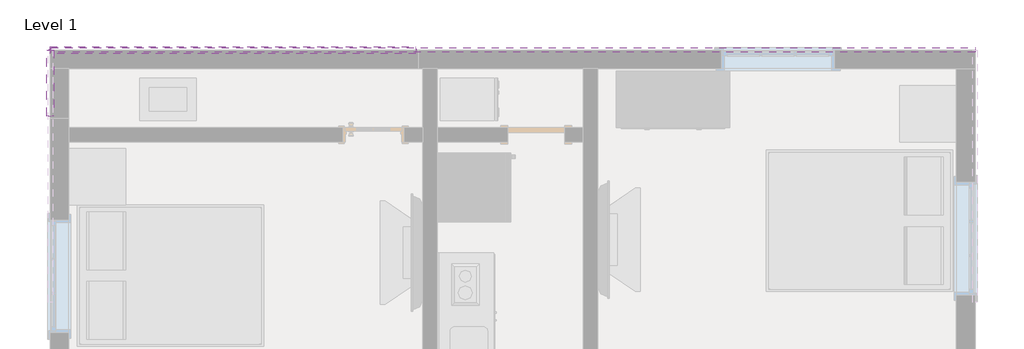
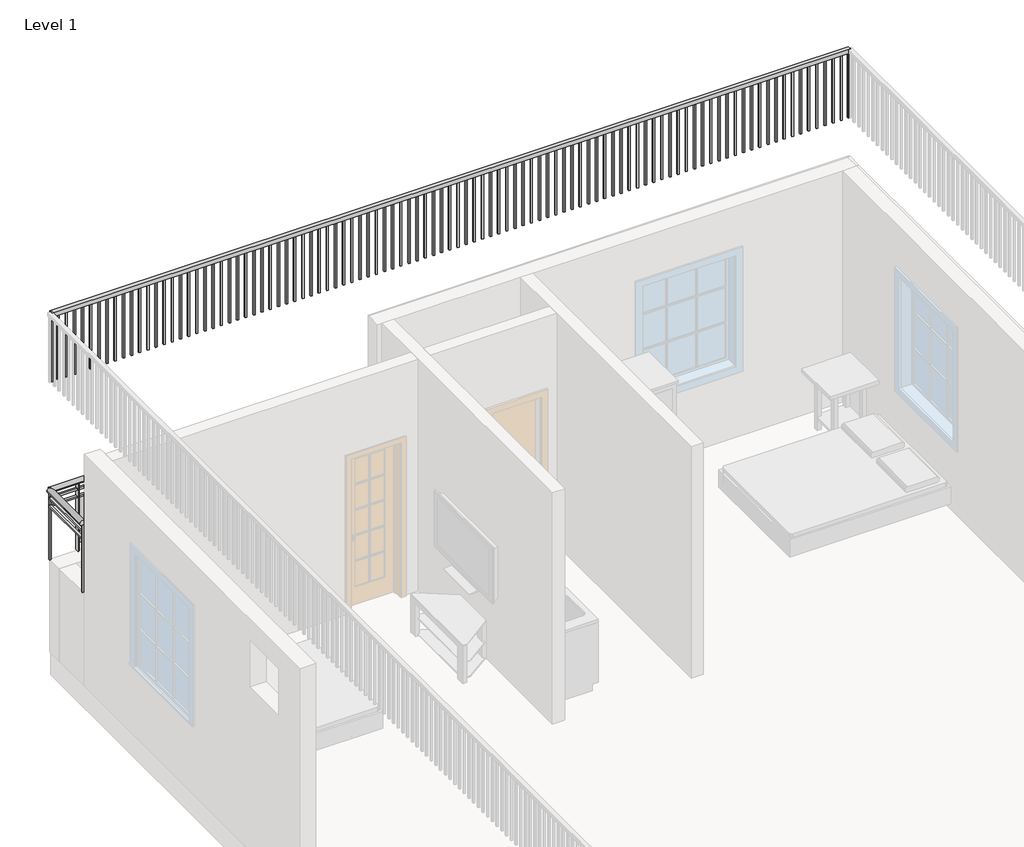
# One storey, part 5 of 7: 3 railings.
"""IFC4 building model written with IfcOpenShell, lengths in millimetres."""

from ifc_helpers import new_model, si_unit, point, frame, origin, place, context, project, spatial, polyline, ellipse_curve, trimmed, outline, extrude, element, save
from ifc_brep_helpers import plane_surface, extruded_surface, advanced_brep

model = new_model("IFC4")

# Units and contexts
model_context = context("Model", 3, world=origin())
ifc_project = project(units=[si_unit("LENGTHUNIT", "METRE", prefix="MILLI")], contexts=[model_context])

# Site, building, storey
site = spatial("IfcSite", under=ifc_project)
building = spatial("IfcBuilding", under=site)
storey = spatial("IfcBuildingStorey", under=building, Name="Level 1", Elevation=0.0)

# Railings
placement = place(None, origin())
element("IfcRailing", 1, ObjectType="Glass Panel - Bottom Fill", at=placement, inside=storey, context=model_context, shape_type="SolidModel", body=[
    advanced_brep(
    [(-4543.28475, 12412.5839473, 2133.6), (-4543.28475, 12488.7839473, 2133.6), (-8480.28475, 12412.5839473, 2133.6), (-8480.28475, 12488.7839473, 2133.6)],
    [
        (0, 1, ellipse_curve(frame((-4543.28475, 12450.6839473, 2133.6), z_axis=(1.0, 0.0, 0.0), x_axis=(0.0, 1.0, 0.0)), 38.1, 28.575)),
        (1, 0, ellipse_curve(frame((-4543.28475, 12450.6839473, 2133.6), z_axis=(1.0, 0.0, 0.0), x_axis=(0.0, 1.0, 0.0)), 38.1, 28.575)),
        (2, 3, ellipse_curve(frame((-8480.28475, 12450.6839473, 2133.6), z_axis=(-1.0, 0.0, 0.0), x_axis=(0.0, 1.0, 0.0)), 38.1, 28.575)),
        (3, 2, ellipse_curve(frame((-8480.28475, 12450.6839473, 2133.6), z_axis=(-1.0, 0.0, 0.0), x_axis=(0.0, 1.0, 0.0)), 38.1, 28.575)),
        (0, 2),
        (3, 1),
    ],
    [
        plane_surface(frame((-4543.28475, 12450.6839473, 2133.6), z_axis=(1.0, 0.0, 0.0), x_axis=(0.0, -1.0, 0.0))),
        plane_surface(frame((-8480.28475, 12450.6839473, 2133.6), z_axis=(-1.0, 0.0, 0.0), x_axis=(0.0, -1.0, 0.0))),
        extruded_surface(trimmed(ellipse_curve(frame((-8480.28475, 12450.6839473, 2133.6), z_axis=(1.0, 0.0, 0.0), x_axis=(0.0, 1.0, 0.0)), 38.1, 28.575), [point((-8480.28475, 12412.5839473, 2133.6))], [point((-8480.28475, 12488.7839473, 2133.6))], True, "CARTESIAN"), (3937.000000000001, 0.0, 0.0), 3937.000000000001),
        extruded_surface(trimmed(ellipse_curve(frame((-8480.28475, 12450.6839473, 2133.6), z_axis=(1.0, 0.0, 0.0), x_axis=(0.0, 1.0, 0.0)), 38.1, 28.575), [point((-8480.28475, 12488.7839473, 2133.6))], [point((-8480.28475, 12412.5839473, 2133.6))], True, "CARTESIAN"), (3937.000000000001, 0.0, 0.0), 3937.000000000001),
    ],
    [
        (0, [[1, 2]]),
        (1, [[3, 4]]),
        (2, [[-1, 5, -4, 6]]),
        (3, [[-2, -6, -3, -5]]),
    ],
),
    extrude(outline(polyline([(-4543.28475, 12463.3839473), (-4543.28475, 12437.9839473), (-8480.28475, 12437.9839473), (-8480.28475, 12463.3839473), (-4543.28475, 12463.3839473)])), frame((0.0, 0.0, 2019.3), z_axis=(0.0, 0.0, 1.0), x_axis=(1.0, 0.0, 0.0)), (0.0, 0.0, 1.0), 25.4),
    extrude(outline(polyline([(-4543.28475, 12463.3839473), (-4543.28475, 12437.9839473), (-8480.28475, 12437.9839473), (-8480.28475, 12463.3839473), (-4543.28475, 12463.3839473)])), frame((0.0, 0.0, 1917.7), z_axis=(0.0, 0.0, 1.0), x_axis=(1.0, 0.0, 0.0)), (0.0, 0.0, 1.0), 25.4),
    extrude(outline(polyline([(-8131.03475, 12476.0839473), (-8131.03475, 12425.2839473), (-8143.73475, 12425.2839473), (-8143.73475, 12476.0839473), (-8131.03475, 12476.0839473)])), frame((0.0, 0.0, 1219.2), z_axis=(0.0, 0.0, 1.0), x_axis=(1.0, 0.0, 0.0)), (0.0, 0.0, 1.0), 885.6788223),
    extrude(outline(polyline([(-7324.58475, 12444.1487903), (-8137.38475, 12444.1487903), (-8137.38475, 12450.4987903), (-7324.58475, 12450.4987903), (-7324.58475, 12444.1487903)])), frame((0.0, 0.0, 1320.8), z_axis=(0.0, 0.0, 1.0), x_axis=(1.0, 0.0, 0.0)), (0.0, 0.0, 1.0), 596.9),
    extrude(outline(polyline([(-7318.23475, 12476.0839473), (-7318.23475, 12425.2839473), (-7330.93475, 12425.2839473), (-7330.93475, 12476.0839473), (-7318.23475, 12476.0839473)])), frame((0.0, 0.0, 1219.2), z_axis=(0.0, 0.0, 1.0), x_axis=(1.0, 0.0, 0.0)), (0.0, 0.0, 1.0), 885.6788223),
    extrude(outline(polyline([(-6511.78475, 12444.1487903), (-7324.58475, 12444.1487903), (-7324.58475, 12450.4987903), (-6511.78475, 12450.4987903), (-6511.78475, 12444.1487903)])), frame((0.0, 0.0, 1320.8), z_axis=(0.0, 0.0, 1.0), x_axis=(1.0, 0.0, 0.0)), (0.0, 0.0, 1.0), 596.9),
    extrude(outline(polyline([(-6505.43475, 12476.0839473), (-6505.43475, 12425.2839473), (-6518.13475, 12425.2839473), (-6518.13475, 12476.0839473), (-6505.43475, 12476.0839473)])), frame((0.0, 0.0, 1219.2), z_axis=(0.0, 0.0, 1.0), x_axis=(1.0, 0.0, 0.0)), (0.0, 0.0, 1.0), 885.6788223),
    extrude(outline(polyline([(-5698.98475, 12444.1487903), (-6511.78475, 12444.1487903), (-6511.78475, 12450.4987903), (-5698.98475, 12450.4987903), (-5698.98475, 12444.1487903)])), frame((0.0, 0.0, 1320.8), z_axis=(0.0, 0.0, 1.0), x_axis=(1.0, 0.0, 0.0)), (0.0, 0.0, 1.0), 596.9),
    extrude(outline(polyline([(-5692.63475, 12476.0839473), (-5692.63475, 12425.2839473), (-5705.33475, 12425.2839473), (-5705.33475, 12476.0839473), (-5692.63475, 12476.0839473)])), frame((0.0, 0.0, 1219.2), z_axis=(0.0, 0.0, 1.0), x_axis=(1.0, 0.0, 0.0)), (0.0, 0.0, 1.0), 885.6788223),
    extrude(outline(polyline([(-4886.18475, 12444.1487903), (-5698.98475, 12444.1487903), (-5698.98475, 12450.4987903), (-4886.18475, 12450.4987903), (-4886.18475, 12444.1487903)])), frame((0.0, 0.0, 1320.8), z_axis=(0.0, 0.0, 1.0), x_axis=(1.0, 0.0, 0.0)), (0.0, 0.0, 1.0), 596.9),
    extrude(outline(polyline([(-4879.83475, 12476.0839473), (-4879.83475, 12425.2839473), (-4892.53475, 12425.2839473), (-4892.53475, 12476.0839473), (-4879.83475, 12476.0839473)])), frame((0.0, 0.0, 1219.2), z_axis=(0.0, 0.0, 1.0), x_axis=(1.0, 0.0, 0.0)), (0.0, 0.0, 1.0), 885.6788223),
    extrude(outline(polyline([(-8467.58475, 12460.2089473), (-8467.58475, 12441.1589473), (-8486.63475, 12441.1589473), (-8486.63475, 12460.2089473), (-8467.58475, 12460.2089473)])), frame((0.0, 0.0, 1219.2), z_axis=(0.0, 0.0, 1.0), x_axis=(1.0, 0.0, 0.0)), (0.0, 0.0, 1.0), 885.6788223),
    extrude(outline(polyline([(-4536.93475, 12460.2089473), (-4536.93475, 12441.1589473), (-4555.98475, 12441.1589473), (-4555.98475, 12460.2089473), (-4536.93475, 12460.2089473)])), frame((0.0, 0.0, 1219.2), z_axis=(0.0, 0.0, 1.0), x_axis=(1.0, 0.0, 0.0)), (0.0, 0.0, 1.0), 885.6788223),
])
element("IfcRailing", 2, ObjectType="Glass Panel - Bottom Fill", at=placement, inside=storey, context=model_context, shape_type="SolidModel", body=[
    advanced_brep(
    [(-8442.18475, 12450.6839473, 2133.6), (-8518.38475, 12450.6839473, 2133.6), (-8442.18475, 11739.4839473, 2133.6), (-8518.38475, 11739.4839473, 2133.6)],
    [
        (0, 1, ellipse_curve(frame((-8480.28475, 12450.6839473, 2133.6), z_axis=(0.0, 1.0, 0.0), x_axis=(-1.0, 0.0, 0.0)), 38.1, 28.575)),
        (1, 0, ellipse_curve(frame((-8480.28475, 12450.6839473, 2133.6), z_axis=(0.0, 1.0, 0.0), x_axis=(-1.0, 0.0, 0.0)), 38.1, 28.575)),
        (2, 3, ellipse_curve(frame((-8480.28475, 11739.4839473, 2133.6), z_axis=(0.0, -1.0, 0.0), x_axis=(-1.0, 0.0, 0.0)), 38.1, 28.575)),
        (3, 2, ellipse_curve(frame((-8480.28475, 11739.4839473, 2133.6), z_axis=(0.0, -1.0, 0.0), x_axis=(-1.0, 0.0, 0.0)), 38.1, 28.575)),
        (0, 2),
        (3, 1),
    ],
    [
        plane_surface(frame((-8480.28475, 12450.6839473, 2133.6), z_axis=(0.0, 1.0, 0.0), x_axis=(0.0, 0.0, -1.0))),
        plane_surface(frame((-8480.28475, 11739.4839473, 2133.6), z_axis=(0.0, -1.0, 0.0), x_axis=(0.0, 0.0, -1.0))),
        extruded_surface(trimmed(ellipse_curve(frame((-8480.28475, 11739.4839473, 2133.6), z_axis=(0.0, 1.0, 0.0), x_axis=(-1.0, 0.0, 0.0)), 38.1, 28.575), [point((-8442.18475, 11739.4839473, 2133.6))], [point((-8518.38475, 11739.4839473, 2133.6))], True, "CARTESIAN"), (0.0, 711.2000000000007, 0.0), 711.2000000000007),
        extruded_surface(trimmed(ellipse_curve(frame((-8480.28475, 11739.4839473, 2133.6), z_axis=(0.0, 1.0, 0.0), x_axis=(-1.0, 0.0, 0.0)), 38.1, 28.575), [point((-8518.38475, 11739.4839473, 2133.6))], [point((-8442.18475, 11739.4839473, 2133.6))], True, "CARTESIAN"), (0.0, 711.2000000000007, 0.0), 711.2000000000007),
    ],
    [
        (0, [[1, 2]]),
        (1, [[3, 4]]),
        (2, [[-1, 5, -4, 6]]),
        (3, [[-2, -6, -3, -5]]),
    ],
),
    extrude(outline(polyline([(-8492.98475, 12450.6839473), (-8467.58475, 12450.6839473), (-8467.58475, 11739.4839473), (-8492.98475, 11739.4839473), (-8492.98475, 12450.6839473)])), frame((0.0, 0.0, 2019.3), z_axis=(0.0, 0.0, 1.0), x_axis=(1.0, 0.0, 0.0)), (0.0, 0.0, 1.0), 25.4),
    extrude(outline(polyline([(-8492.98475, 12450.6839473), (-8467.58475, 12450.6839473), (-8467.58475, 11739.4839473), (-8492.98475, 11739.4839473), (-8492.98475, 12450.6839473)])), frame((0.0, 0.0, 1917.7), z_axis=(0.0, 0.0, 1.0), x_axis=(1.0, 0.0, 0.0)), (0.0, 0.0, 1.0), 25.4),
    extrude(outline(polyline([(-8489.80975, 11752.1839473), (-8470.75975, 11752.1839473), (-8470.75975, 11733.1339473), (-8489.80975, 11733.1339473), (-8489.80975, 11752.1839473)])), frame((0.0, 0.0, 1219.2), z_axis=(0.0, 0.0, 1.0), x_axis=(1.0, 0.0, 0.0)), (0.0, 0.0, 1.0), 885.6788223),
    extrude(outline(polyline([(-8489.80975, 12457.0339473), (-8470.75975, 12457.0339473), (-8470.75975, 12437.9839473), (-8489.80975, 12437.9839473), (-8489.80975, 12457.0339473)])), frame((0.0, 0.0, 1219.2), z_axis=(0.0, 0.0, 1.0), x_axis=(1.0, 0.0, 0.0)), (0.0, 0.0, 1.0), 885.6788223),
])
element("IfcRailing", 3, ObjectType="Handrail - Rectangular", at=placement, inside=storey, context=model_context, shape_type="SweptSolid", body=[
    extrude(outline(polyline([(1476.51525, 12476.0839473), (1476.51525, 12425.2839473), (-8467.58475, 12425.2839473), (-8467.58475, 12476.0839473), (1476.51525, 12476.0839473)])), frame((0.0, 0.0, 4419.6), z_axis=(0.0, 0.0, 1.0), x_axis=(1.0, 0.0, 0.0)), (0.0, 0.0, 1.0), 50.8),
    extrude(outline(polyline([(-8369.15975, 12460.2089473), (-8369.15975, 12441.1589473), (-8388.20975, 12441.1589473), (-8388.20975, 12460.2089473), (-8369.15975, 12460.2089473)])), frame((0.0, 0.0, 3556.0), z_axis=(0.0, 0.0, 1.0), x_axis=(1.0, 0.0, 0.0)), (0.0, 0.0, 1.0), 863.6),
    extrude(outline(polyline([(-8267.55975, 12460.2089473), (-8267.55975, 12441.1589473), (-8286.60975, 12441.1589473), (-8286.60975, 12460.2089473), (-8267.55975, 12460.2089473)])), frame((0.0, 0.0, 3556.0), z_axis=(0.0, 0.0, 1.0), x_axis=(1.0, 0.0, 0.0)), (0.0, 0.0, 1.0), 863.6),
    extrude(outline(polyline([(-8165.95975, 12460.2089473), (-8165.95975, 12441.1589473), (-8185.00975, 12441.1589473), (-8185.00975, 12460.2089473), (-8165.95975, 12460.2089473)])), frame((0.0, 0.0, 3556.0), z_axis=(0.0, 0.0, 1.0), x_axis=(1.0, 0.0, 0.0)), (0.0, 0.0, 1.0), 863.6),
    extrude(outline(polyline([(-8064.35975, 12460.2089473), (-8064.35975, 12441.1589473), (-8083.40975, 12441.1589473), (-8083.40975, 12460.2089473), (-8064.35975, 12460.2089473)])), frame((0.0, 0.0, 3556.0), z_axis=(0.0, 0.0, 1.0), x_axis=(1.0, 0.0, 0.0)), (0.0, 0.0, 1.0), 863.6),
    extrude(outline(polyline([(-7962.75975, 12460.2089473), (-7962.75975, 12441.1589473), (-7981.80975, 12441.1589473), (-7981.80975, 12460.2089473), (-7962.75975, 12460.2089473)])), frame((0.0, 0.0, 3556.0), z_axis=(0.0, 0.0, 1.0), x_axis=(1.0, 0.0, 0.0)), (0.0, 0.0, 1.0), 863.6),
    extrude(outline(polyline([(-7861.15975, 12460.2089473), (-7861.15975, 12441.1589473), (-7880.20975, 12441.1589473), (-7880.20975, 12460.2089473), (-7861.15975, 12460.2089473)])), frame((0.0, 0.0, 3556.0), z_axis=(0.0, 0.0, 1.0), x_axis=(1.0, 0.0, 0.0)), (0.0, 0.0, 1.0), 863.6),
    extrude(outline(polyline([(-7759.55975, 12460.2089473), (-7759.55975, 12441.1589473), (-7778.60975, 12441.1589473), (-7778.60975, 12460.2089473), (-7759.55975, 12460.2089473)])), frame((0.0, 0.0, 3556.0), z_axis=(0.0, 0.0, 1.0), x_axis=(1.0, 0.0, 0.0)), (0.0, 0.0, 1.0), 863.6),
    extrude(outline(polyline([(-7657.95975, 12460.2089473), (-7657.95975, 12441.1589473), (-7677.00975, 12441.1589473), (-7677.00975, 12460.2089473), (-7657.95975, 12460.2089473)])), frame((0.0, 0.0, 3556.0), z_axis=(0.0, 0.0, 1.0), x_axis=(1.0, 0.0, 0.0)), (0.0, 0.0, 1.0), 863.6),
    extrude(outline(polyline([(-7556.35975, 12460.2089473), (-7556.35975, 12441.1589473), (-7575.40975, 12441.1589473), (-7575.40975, 12460.2089473), (-7556.35975, 12460.2089473)])), frame((0.0, 0.0, 3556.0), z_axis=(0.0, 0.0, 1.0), x_axis=(1.0, 0.0, 0.0)), (0.0, 0.0, 1.0), 863.6),
    extrude(outline(polyline([(-7454.75975, 12460.2089473), (-7454.75975, 12441.1589473), (-7473.80975, 12441.1589473), (-7473.80975, 12460.2089473), (-7454.75975, 12460.2089473)])), frame((0.0, 0.0, 3556.0), z_axis=(0.0, 0.0, 1.0), x_axis=(1.0, 0.0, 0.0)), (0.0, 0.0, 1.0), 863.6),
    extrude(outline(polyline([(-7353.15975, 12460.2089473), (-7353.15975, 12441.1589473), (-7372.20975, 12441.1589473), (-7372.20975, 12460.2089473), (-7353.15975, 12460.2089473)])), frame((0.0, 0.0, 3556.0), z_axis=(0.0, 0.0, 1.0), x_axis=(1.0, 0.0, 0.0)), (0.0, 0.0, 1.0), 863.6),
    extrude(outline(polyline([(-7251.55975, 12460.2089473), (-7251.55975, 12441.1589473), (-7270.60975, 12441.1589473), (-7270.60975, 12460.2089473), (-7251.55975, 12460.2089473)])), frame((0.0, 0.0, 3556.0), z_axis=(0.0, 0.0, 1.0), x_axis=(1.0, 0.0, 0.0)), (0.0, 0.0, 1.0), 863.6),
    extrude(outline(polyline([(-7149.95975, 12460.2089473), (-7149.95975, 12441.1589473), (-7169.00975, 12441.1589473), (-7169.00975, 12460.2089473), (-7149.95975, 12460.2089473)])), frame((0.0, 0.0, 3556.0), z_axis=(0.0, 0.0, 1.0), x_axis=(1.0, 0.0, 0.0)), (0.0, 0.0, 1.0), 863.6),
    extrude(outline(polyline([(-7048.35975, 12460.2089473), (-7048.35975, 12441.1589473), (-7067.40975, 12441.1589473), (-7067.40975, 12460.2089473), (-7048.35975, 12460.2089473)])), frame((0.0, 0.0, 3556.0), z_axis=(0.0, 0.0, 1.0), x_axis=(1.0, 0.0, 0.0)), (0.0, 0.0, 1.0), 863.6),
    extrude(outline(polyline([(-6946.75975, 12460.2089473), (-6946.75975, 12441.1589473), (-6965.80975, 12441.1589473), (-6965.80975, 12460.2089473), (-6946.75975, 12460.2089473)])), frame((0.0, 0.0, 3556.0), z_axis=(0.0, 0.0, 1.0), x_axis=(1.0, 0.0, 0.0)), (0.0, 0.0, 1.0), 863.6),
    extrude(outline(polyline([(-6845.15975, 12460.2089473), (-6845.15975, 12441.1589473), (-6864.20975, 12441.1589473), (-6864.20975, 12460.2089473), (-6845.15975, 12460.2089473)])), frame((0.0, 0.0, 3556.0), z_axis=(0.0, 0.0, 1.0), x_axis=(1.0, 0.0, 0.0)), (0.0, 0.0, 1.0), 863.6),
    extrude(outline(polyline([(-6743.55975, 12460.2089473), (-6743.55975, 12441.1589473), (-6762.60975, 12441.1589473), (-6762.60975, 12460.2089473), (-6743.55975, 12460.2089473)])), frame((0.0, 0.0, 3556.0), z_axis=(0.0, 0.0, 1.0), x_axis=(1.0, 0.0, 0.0)), (0.0, 0.0, 1.0), 863.6),
    extrude(outline(polyline([(-6641.95975, 12460.2089473), (-6641.95975, 12441.1589473), (-6661.00975, 12441.1589473), (-6661.00975, 12460.2089473), (-6641.95975, 12460.2089473)])), frame((0.0, 0.0, 3556.0), z_axis=(0.0, 0.0, 1.0), x_axis=(1.0, 0.0, 0.0)), (0.0, 0.0, 1.0), 863.6),
    extrude(outline(polyline([(-6540.35975, 12460.2089473), (-6540.35975, 12441.1589473), (-6559.40975, 12441.1589473), (-6559.40975, 12460.2089473), (-6540.35975, 12460.2089473)])), frame((0.0, 0.0, 3556.0), z_axis=(0.0, 0.0, 1.0), x_axis=(1.0, 0.0, 0.0)), (0.0, 0.0, 1.0), 863.6),
    extrude(outline(polyline([(-6438.75975, 12460.2089473), (-6438.75975, 12441.1589473), (-6457.80975, 12441.1589473), (-6457.80975, 12460.2089473), (-6438.75975, 12460.2089473)])), frame((0.0, 0.0, 3556.0), z_axis=(0.0, 0.0, 1.0), x_axis=(1.0, 0.0, 0.0)), (0.0, 0.0, 1.0), 863.6),
    extrude(outline(polyline([(-6337.15975, 12460.2089473), (-6337.15975, 12441.1589473), (-6356.20975, 12441.1589473), (-6356.20975, 12460.2089473), (-6337.15975, 12460.2089473)])), frame((0.0, 0.0, 3556.0), z_axis=(0.0, 0.0, 1.0), x_axis=(1.0, 0.0, 0.0)), (0.0, 0.0, 1.0), 863.6),
    extrude(outline(polyline([(-6235.55975, 12460.2089473), (-6235.55975, 12441.1589473), (-6254.60975, 12441.1589473), (-6254.60975, 12460.2089473), (-6235.55975, 12460.2089473)])), frame((0.0, 0.0, 3556.0), z_axis=(0.0, 0.0, 1.0), x_axis=(1.0, 0.0, 0.0)), (0.0, 0.0, 1.0), 863.6),
    extrude(outline(polyline([(-6133.95975, 12460.2089473), (-6133.95975, 12441.1589473), (-6153.00975, 12441.1589473), (-6153.00975, 12460.2089473), (-6133.95975, 12460.2089473)])), frame((0.0, 0.0, 3556.0), z_axis=(0.0, 0.0, 1.0), x_axis=(1.0, 0.0, 0.0)), (0.0, 0.0, 1.0), 863.6),
    extrude(outline(polyline([(-6032.35975, 12460.2089473), (-6032.35975, 12441.1589473), (-6051.40975, 12441.1589473), (-6051.40975, 12460.2089473), (-6032.35975, 12460.2089473)])), frame((0.0, 0.0, 3556.0), z_axis=(0.0, 0.0, 1.0), x_axis=(1.0, 0.0, 0.0)), (0.0, 0.0, 1.0), 863.6),
    extrude(outline(polyline([(-5930.75975, 12460.2089473), (-5930.75975, 12441.1589473), (-5949.80975, 12441.1589473), (-5949.80975, 12460.2089473), (-5930.75975, 12460.2089473)])), frame((0.0, 0.0, 3556.0), z_axis=(0.0, 0.0, 1.0), x_axis=(1.0, 0.0, 0.0)), (0.0, 0.0, 1.0), 863.6),
    extrude(outline(polyline([(-5829.15975, 12460.2089473), (-5829.15975, 12441.1589473), (-5848.20975, 12441.1589473), (-5848.20975, 12460.2089473), (-5829.15975, 12460.2089473)])), frame((0.0, 0.0, 3556.0), z_axis=(0.0, 0.0, 1.0), x_axis=(1.0, 0.0, 0.0)), (0.0, 0.0, 1.0), 863.6),
    extrude(outline(polyline([(-5727.55975, 12460.2089473), (-5727.55975, 12441.1589473), (-5746.60975, 12441.1589473), (-5746.60975, 12460.2089473), (-5727.55975, 12460.2089473)])), frame((0.0, 0.0, 3556.0), z_axis=(0.0, 0.0, 1.0), x_axis=(1.0, 0.0, 0.0)), (0.0, 0.0, 1.0), 863.6),
    extrude(outline(polyline([(-5625.95975, 12460.2089473), (-5625.95975, 12441.1589473), (-5645.00975, 12441.1589473), (-5645.00975, 12460.2089473), (-5625.95975, 12460.2089473)])), frame((0.0, 0.0, 3556.0), z_axis=(0.0, 0.0, 1.0), x_axis=(1.0, 0.0, 0.0)), (0.0, 0.0, 1.0), 863.6),
    extrude(outline(polyline([(-5524.35975, 12460.2089473), (-5524.35975, 12441.1589473), (-5543.40975, 12441.1589473), (-5543.40975, 12460.2089473), (-5524.35975, 12460.2089473)])), frame((0.0, 0.0, 3556.0), z_axis=(0.0, 0.0, 1.0), x_axis=(1.0, 0.0, 0.0)), (0.0, 0.0, 1.0), 863.6),
    extrude(outline(polyline([(-5422.75975, 12460.2089473), (-5422.75975, 12441.1589473), (-5441.80975, 12441.1589473), (-5441.80975, 12460.2089473), (-5422.75975, 12460.2089473)])), frame((0.0, 0.0, 3556.0), z_axis=(0.0, 0.0, 1.0), x_axis=(1.0, 0.0, 0.0)), (0.0, 0.0, 1.0), 863.6),
    extrude(outline(polyline([(-5321.15975, 12460.2089473), (-5321.15975, 12441.1589473), (-5340.20975, 12441.1589473), (-5340.20975, 12460.2089473), (-5321.15975, 12460.2089473)])), frame((0.0, 0.0, 3556.0), z_axis=(0.0, 0.0, 1.0), x_axis=(1.0, 0.0, 0.0)), (0.0, 0.0, 1.0), 863.6),
    extrude(outline(polyline([(-5219.55975, 12460.2089473), (-5219.55975, 12441.1589473), (-5238.60975, 12441.1589473), (-5238.60975, 12460.2089473), (-5219.55975, 12460.2089473)])), frame((0.0, 0.0, 3556.0), z_axis=(0.0, 0.0, 1.0), x_axis=(1.0, 0.0, 0.0)), (0.0, 0.0, 1.0), 863.6),
    extrude(outline(polyline([(-5117.95975, 12460.2089473), (-5117.95975, 12441.1589473), (-5137.00975, 12441.1589473), (-5137.00975, 12460.2089473), (-5117.95975, 12460.2089473)])), frame((0.0, 0.0, 3556.0), z_axis=(0.0, 0.0, 1.0), x_axis=(1.0, 0.0, 0.0)), (0.0, 0.0, 1.0), 863.6),
    extrude(outline(polyline([(-5016.35975, 12460.2089473), (-5016.35975, 12441.1589473), (-5035.40975, 12441.1589473), (-5035.40975, 12460.2089473), (-5016.35975, 12460.2089473)])), frame((0.0, 0.0, 3556.0), z_axis=(0.0, 0.0, 1.0), x_axis=(1.0, 0.0, 0.0)), (0.0, 0.0, 1.0), 863.6),
    extrude(outline(polyline([(-4914.75975, 12460.2089473), (-4914.75975, 12441.1589473), (-4933.80975, 12441.1589473), (-4933.80975, 12460.2089473), (-4914.75975, 12460.2089473)])), frame((0.0, 0.0, 3556.0), z_axis=(0.0, 0.0, 1.0), x_axis=(1.0, 0.0, 0.0)), (0.0, 0.0, 1.0), 863.6),
    extrude(outline(polyline([(-4813.15975, 12460.2089473), (-4813.15975, 12441.1589473), (-4832.20975, 12441.1589473), (-4832.20975, 12460.2089473), (-4813.15975, 12460.2089473)])), frame((0.0, 0.0, 3556.0), z_axis=(0.0, 0.0, 1.0), x_axis=(1.0, 0.0, 0.0)), (0.0, 0.0, 1.0), 863.6),
    extrude(outline(polyline([(-4711.55975, 12460.2089473), (-4711.55975, 12441.1589473), (-4730.60975, 12441.1589473), (-4730.60975, 12460.2089473), (-4711.55975, 12460.2089473)])), frame((0.0, 0.0, 3556.0), z_axis=(0.0, 0.0, 1.0), x_axis=(1.0, 0.0, 0.0)), (0.0, 0.0, 1.0), 863.6),
    extrude(outline(polyline([(-4609.95975, 12460.2089473), (-4609.95975, 12441.1589473), (-4629.00975, 12441.1589473), (-4629.00975, 12460.2089473), (-4609.95975, 12460.2089473)])), frame((0.0, 0.0, 3556.0), z_axis=(0.0, 0.0, 1.0), x_axis=(1.0, 0.0, 0.0)), (0.0, 0.0, 1.0), 863.6),
    extrude(outline(polyline([(-4508.35975, 12460.2089473), (-4508.35975, 12441.1589473), (-4527.40975, 12441.1589473), (-4527.40975, 12460.2089473), (-4508.35975, 12460.2089473)])), frame((0.0, 0.0, 3556.0), z_axis=(0.0, 0.0, 1.0), x_axis=(1.0, 0.0, 0.0)), (0.0, 0.0, 1.0), 863.6),
    extrude(outline(polyline([(-4406.75975, 12460.2089473), (-4406.75975, 12441.1589473), (-4425.80975, 12441.1589473), (-4425.80975, 12460.2089473), (-4406.75975, 12460.2089473)])), frame((0.0, 0.0, 3556.0), z_axis=(0.0, 0.0, 1.0), x_axis=(1.0, 0.0, 0.0)), (0.0, 0.0, 1.0), 863.6),
    extrude(outline(polyline([(-4305.15975, 12460.2089473), (-4305.15975, 12441.1589473), (-4324.20975, 12441.1589473), (-4324.20975, 12460.2089473), (-4305.15975, 12460.2089473)])), frame((0.0, 0.0, 3556.0), z_axis=(0.0, 0.0, 1.0), x_axis=(1.0, 0.0, 0.0)), (0.0, 0.0, 1.0), 863.6),
    extrude(outline(polyline([(-4203.55975, 12460.2089473), (-4203.55975, 12441.1589473), (-4222.60975, 12441.1589473), (-4222.60975, 12460.2089473), (-4203.55975, 12460.2089473)])), frame((0.0, 0.0, 3556.0), z_axis=(0.0, 0.0, 1.0), x_axis=(1.0, 0.0, 0.0)), (0.0, 0.0, 1.0), 863.6),
    extrude(outline(polyline([(-4101.95975, 12460.2089473), (-4101.95975, 12441.1589473), (-4121.00975, 12441.1589473), (-4121.00975, 12460.2089473), (-4101.95975, 12460.2089473)])), frame((0.0, 0.0, 3556.0), z_axis=(0.0, 0.0, 1.0), x_axis=(1.0, 0.0, 0.0)), (0.0, 0.0, 1.0), 863.6),
    extrude(outline(polyline([(-4000.35975, 12460.2089473), (-4000.35975, 12441.1589473), (-4019.40975, 12441.1589473), (-4019.40975, 12460.2089473), (-4000.35975, 12460.2089473)])), frame((0.0, 0.0, 3556.0), z_axis=(0.0, 0.0, 1.0), x_axis=(1.0, 0.0, 0.0)), (0.0, 0.0, 1.0), 863.6),
    extrude(outline(polyline([(-3898.75975, 12460.2089473), (-3898.75975, 12441.1589473), (-3917.80975, 12441.1589473), (-3917.80975, 12460.2089473), (-3898.75975, 12460.2089473)])), frame((0.0, 0.0, 3556.0), z_axis=(0.0, 0.0, 1.0), x_axis=(1.0, 0.0, 0.0)), (0.0, 0.0, 1.0), 863.6),
    extrude(outline(polyline([(-3797.15975, 12460.2089473), (-3797.15975, 12441.1589473), (-3816.20975, 12441.1589473), (-3816.20975, 12460.2089473), (-3797.15975, 12460.2089473)])), frame((0.0, 0.0, 3556.0), z_axis=(0.0, 0.0, 1.0), x_axis=(1.0, 0.0, 0.0)), (0.0, 0.0, 1.0), 863.6),
    extrude(outline(polyline([(-3695.55975, 12460.2089473), (-3695.55975, 12441.1589473), (-3714.60975, 12441.1589473), (-3714.60975, 12460.2089473), (-3695.55975, 12460.2089473)])), frame((0.0, 0.0, 3556.0), z_axis=(0.0, 0.0, 1.0), x_axis=(1.0, 0.0, 0.0)), (0.0, 0.0, 1.0), 863.6),
    extrude(outline(polyline([(-3593.95975, 12460.2089473), (-3593.95975, 12441.1589473), (-3613.00975, 12441.1589473), (-3613.00975, 12460.2089473), (-3593.95975, 12460.2089473)])), frame((0.0, 0.0, 3556.0), z_axis=(0.0, 0.0, 1.0), x_axis=(1.0, 0.0, 0.0)), (0.0, 0.0, 1.0), 863.6),
    extrude(outline(polyline([(-3492.35975, 12460.2089473), (-3492.35975, 12441.1589473), (-3511.40975, 12441.1589473), (-3511.40975, 12460.2089473), (-3492.35975, 12460.2089473)])), frame((0.0, 0.0, 3556.0), z_axis=(0.0, 0.0, 1.0), x_axis=(1.0, 0.0, 0.0)), (0.0, 0.0, 1.0), 863.6),
    extrude(outline(polyline([(-3390.75975, 12460.2089473), (-3390.75975, 12441.1589473), (-3409.80975, 12441.1589473), (-3409.80975, 12460.2089473), (-3390.75975, 12460.2089473)])), frame((0.0, 0.0, 3556.0), z_axis=(0.0, 0.0, 1.0), x_axis=(1.0, 0.0, 0.0)), (0.0, 0.0, 1.0), 863.6),
    extrude(outline(polyline([(-3289.15975, 12460.2089473), (-3289.15975, 12441.1589473), (-3308.20975, 12441.1589473), (-3308.20975, 12460.2089473), (-3289.15975, 12460.2089473)])), frame((0.0, 0.0, 3556.0), z_axis=(0.0, 0.0, 1.0), x_axis=(1.0, 0.0, 0.0)), (0.0, 0.0, 1.0), 863.6),
    extrude(outline(polyline([(-3187.55975, 12460.2089473), (-3187.55975, 12441.1589473), (-3206.60975, 12441.1589473), (-3206.60975, 12460.2089473), (-3187.55975, 12460.2089473)])), frame((0.0, 0.0, 3556.0), z_axis=(0.0, 0.0, 1.0), x_axis=(1.0, 0.0, 0.0)), (0.0, 0.0, 1.0), 863.6),
    extrude(outline(polyline([(-3085.95975, 12460.2089473), (-3085.95975, 12441.1589473), (-3105.00975, 12441.1589473), (-3105.00975, 12460.2089473), (-3085.95975, 12460.2089473)])), frame((0.0, 0.0, 3556.0), z_axis=(0.0, 0.0, 1.0), x_axis=(1.0, 0.0, 0.0)), (0.0, 0.0, 1.0), 863.6),
    extrude(outline(polyline([(-2984.35975, 12460.2089473), (-2984.35975, 12441.1589473), (-3003.40975, 12441.1589473), (-3003.40975, 12460.2089473), (-2984.35975, 12460.2089473)])), frame((0.0, 0.0, 3556.0), z_axis=(0.0, 0.0, 1.0), x_axis=(1.0, 0.0, 0.0)), (0.0, 0.0, 1.0), 863.6),
    extrude(outline(polyline([(-2882.75975, 12460.2089473), (-2882.75975, 12441.1589473), (-2901.80975, 12441.1589473), (-2901.80975, 12460.2089473), (-2882.75975, 12460.2089473)])), frame((0.0, 0.0, 3556.0), z_axis=(0.0, 0.0, 1.0), x_axis=(1.0, 0.0, 0.0)), (0.0, 0.0, 1.0), 863.6),
    extrude(outline(polyline([(-2781.15975, 12460.2089473), (-2781.15975, 12441.1589473), (-2800.20975, 12441.1589473), (-2800.20975, 12460.2089473), (-2781.15975, 12460.2089473)])), frame((0.0, 0.0, 3556.0), z_axis=(0.0, 0.0, 1.0), x_axis=(1.0, 0.0, 0.0)), (0.0, 0.0, 1.0), 863.6),
    extrude(outline(polyline([(-2679.55975, 12460.2089473), (-2679.55975, 12441.1589473), (-2698.60975, 12441.1589473), (-2698.60975, 12460.2089473), (-2679.55975, 12460.2089473)])), frame((0.0, 0.0, 3556.0), z_axis=(0.0, 0.0, 1.0), x_axis=(1.0, 0.0, 0.0)), (0.0, 0.0, 1.0), 863.6),
    extrude(outline(polyline([(-2577.95975, 12460.2089473), (-2577.95975, 12441.1589473), (-2597.00975, 12441.1589473), (-2597.00975, 12460.2089473), (-2577.95975, 12460.2089473)])), frame((0.0, 0.0, 3556.0), z_axis=(0.0, 0.0, 1.0), x_axis=(1.0, 0.0, 0.0)), (0.0, 0.0, 1.0), 863.6),
    extrude(outline(polyline([(-2476.35975, 12460.2089473), (-2476.35975, 12441.1589473), (-2495.40975, 12441.1589473), (-2495.40975, 12460.2089473), (-2476.35975, 12460.2089473)])), frame((0.0, 0.0, 3556.0), z_axis=(0.0, 0.0, 1.0), x_axis=(1.0, 0.0, 0.0)), (0.0, 0.0, 1.0), 863.6),
    extrude(outline(polyline([(-2374.75975, 12460.2089473), (-2374.75975, 12441.1589473), (-2393.80975, 12441.1589473), (-2393.80975, 12460.2089473), (-2374.75975, 12460.2089473)])), frame((0.0, 0.0, 3556.0), z_axis=(0.0, 0.0, 1.0), x_axis=(1.0, 0.0, 0.0)), (0.0, 0.0, 1.0), 863.6),
    extrude(outline(polyline([(-2273.15975, 12460.2089473), (-2273.15975, 12441.1589473), (-2292.20975, 12441.1589473), (-2292.20975, 12460.2089473), (-2273.15975, 12460.2089473)])), frame((0.0, 0.0, 3556.0), z_axis=(0.0, 0.0, 1.0), x_axis=(1.0, 0.0, 0.0)), (0.0, 0.0, 1.0), 863.6),
    extrude(outline(polyline([(-2171.55975, 12460.2089473), (-2171.55975, 12441.1589473), (-2190.60975, 12441.1589473), (-2190.60975, 12460.2089473), (-2171.55975, 12460.2089473)])), frame((0.0, 0.0, 3556.0), z_axis=(0.0, 0.0, 1.0), x_axis=(1.0, 0.0, 0.0)), (0.0, 0.0, 1.0), 863.6),
    extrude(outline(polyline([(-2069.95975, 12460.2089473), (-2069.95975, 12441.1589473), (-2089.00975, 12441.1589473), (-2089.00975, 12460.2089473), (-2069.95975, 12460.2089473)])), frame((0.0, 0.0, 3556.0), z_axis=(0.0, 0.0, 1.0), x_axis=(1.0, 0.0, 0.0)), (0.0, 0.0, 1.0), 863.6),
    extrude(outline(polyline([(-1968.35975, 12460.2089473), (-1968.35975, 12441.1589473), (-1987.40975, 12441.1589473), (-1987.40975, 12460.2089473), (-1968.35975, 12460.2089473)])), frame((0.0, 0.0, 3556.0), z_axis=(0.0, 0.0, 1.0), x_axis=(1.0, 0.0, 0.0)), (0.0, 0.0, 1.0), 863.6),
    extrude(outline(polyline([(-1866.75975, 12460.2089473), (-1866.75975, 12441.1589473), (-1885.80975, 12441.1589473), (-1885.80975, 12460.2089473), (-1866.75975, 12460.2089473)])), frame((0.0, 0.0, 3556.0), z_axis=(0.0, 0.0, 1.0), x_axis=(1.0, 0.0, 0.0)), (0.0, 0.0, 1.0), 863.6),
    extrude(outline(polyline([(-1765.15975, 12460.2089473), (-1765.15975, 12441.1589473), (-1784.20975, 12441.1589473), (-1784.20975, 12460.2089473), (-1765.15975, 12460.2089473)])), frame((0.0, 0.0, 3556.0), z_axis=(0.0, 0.0, 1.0), x_axis=(1.0, 0.0, 0.0)), (0.0, 0.0, 1.0), 863.6),
    extrude(outline(polyline([(-1663.55975, 12460.2089473), (-1663.55975, 12441.1589473), (-1682.60975, 12441.1589473), (-1682.60975, 12460.2089473), (-1663.55975, 12460.2089473)])), frame((0.0, 0.0, 3556.0), z_axis=(0.0, 0.0, 1.0), x_axis=(1.0, 0.0, 0.0)), (0.0, 0.0, 1.0), 863.6),
    extrude(outline(polyline([(-1561.95975, 12460.2089473), (-1561.95975, 12441.1589473), (-1581.00975, 12441.1589473), (-1581.00975, 12460.2089473), (-1561.95975, 12460.2089473)])), frame((0.0, 0.0, 3556.0), z_axis=(0.0, 0.0, 1.0), x_axis=(1.0, 0.0, 0.0)), (0.0, 0.0, 1.0), 863.6),
    extrude(outline(polyline([(-1460.35975, 12460.2089473), (-1460.35975, 12441.1589473), (-1479.40975, 12441.1589473), (-1479.40975, 12460.2089473), (-1460.35975, 12460.2089473)])), frame((0.0, 0.0, 3556.0), z_axis=(0.0, 0.0, 1.0), x_axis=(1.0, 0.0, 0.0)), (0.0, 0.0, 1.0), 863.6),
    extrude(outline(polyline([(-1358.75975, 12460.2089473), (-1358.75975, 12441.1589473), (-1377.80975, 12441.1589473), (-1377.80975, 12460.2089473), (-1358.75975, 12460.2089473)])), frame((0.0, 0.0, 3556.0), z_axis=(0.0, 0.0, 1.0), x_axis=(1.0, 0.0, 0.0)), (0.0, 0.0, 1.0), 863.6),
    extrude(outline(polyline([(-1257.15975, 12460.2089473), (-1257.15975, 12441.1589473), (-1276.20975, 12441.1589473), (-1276.20975, 12460.2089473), (-1257.15975, 12460.2089473)])), frame((0.0, 0.0, 3556.0), z_axis=(0.0, 0.0, 1.0), x_axis=(1.0, 0.0, 0.0)), (0.0, 0.0, 1.0), 863.6),
    extrude(outline(polyline([(-1155.55975, 12460.2089473), (-1155.55975, 12441.1589473), (-1174.60975, 12441.1589473), (-1174.60975, 12460.2089473), (-1155.55975, 12460.2089473)])), frame((0.0, 0.0, 3556.0), z_axis=(0.0, 0.0, 1.0), x_axis=(1.0, 0.0, 0.0)), (0.0, 0.0, 1.0), 863.6),
    extrude(outline(polyline([(-1053.95975, 12460.2089473), (-1053.95975, 12441.1589473), (-1073.00975, 12441.1589473), (-1073.00975, 12460.2089473), (-1053.95975, 12460.2089473)])), frame((0.0, 0.0, 3556.0), z_axis=(0.0, 0.0, 1.0), x_axis=(1.0, 0.0, 0.0)), (0.0, 0.0, 1.0), 863.6),
    extrude(outline(polyline([(-952.35975, 12460.2089473), (-952.35975, 12441.1589473), (-971.40975, 12441.1589473), (-971.40975, 12460.2089473), (-952.35975, 12460.2089473)])), frame((0.0, 0.0, 3556.0), z_axis=(0.0, 0.0, 1.0), x_axis=(1.0, 0.0, 0.0)), (0.0, 0.0, 1.0), 863.6),
    extrude(outline(polyline([(-850.75975, 12460.2089473), (-850.75975, 12441.1589473), (-869.80975, 12441.1589473), (-869.80975, 12460.2089473), (-850.75975, 12460.2089473)])), frame((0.0, 0.0, 3556.0), z_axis=(0.0, 0.0, 1.0), x_axis=(1.0, 0.0, 0.0)), (0.0, 0.0, 1.0), 863.6),
    extrude(outline(polyline([(-749.15975, 12460.2089473), (-749.15975, 12441.1589473), (-768.20975, 12441.1589473), (-768.20975, 12460.2089473), (-749.15975, 12460.2089473)])), frame((0.0, 0.0, 3556.0), z_axis=(0.0, 0.0, 1.0), x_axis=(1.0, 0.0, 0.0)), (0.0, 0.0, 1.0), 863.6),
    extrude(outline(polyline([(-647.55975, 12460.2089473), (-647.55975, 12441.1589473), (-666.60975, 12441.1589473), (-666.60975, 12460.2089473), (-647.55975, 12460.2089473)])), frame((0.0, 0.0, 3556.0), z_axis=(0.0, 0.0, 1.0), x_axis=(1.0, 0.0, 0.0)), (0.0, 0.0, 1.0), 863.6),
    extrude(outline(polyline([(-545.95975, 12460.2089473), (-545.95975, 12441.1589473), (-565.00975, 12441.1589473), (-565.00975, 12460.2089473), (-545.95975, 12460.2089473)])), frame((0.0, 0.0, 3556.0), z_axis=(0.0, 0.0, 1.0), x_axis=(1.0, 0.0, 0.0)), (0.0, 0.0, 1.0), 863.6),
    extrude(outline(polyline([(-444.35975, 12460.2089473), (-444.35975, 12441.1589473), (-463.40975, 12441.1589473), (-463.40975, 12460.2089473), (-444.35975, 12460.2089473)])), frame((0.0, 0.0, 3556.0), z_axis=(0.0, 0.0, 1.0), x_axis=(1.0, 0.0, 0.0)), (0.0, 0.0, 1.0), 863.6),
    extrude(outline(polyline([(-342.75975, 12460.2089473), (-342.75975, 12441.1589473), (-361.80975, 12441.1589473), (-361.80975, 12460.2089473), (-342.75975, 12460.2089473)])), frame((0.0, 0.0, 3556.0), z_axis=(0.0, 0.0, 1.0), x_axis=(1.0, 0.0, 0.0)), (0.0, 0.0, 1.0), 863.6),
    extrude(outline(polyline([(-241.15975, 12460.2089473), (-241.15975, 12441.1589473), (-260.20975, 12441.1589473), (-260.20975, 12460.2089473), (-241.15975, 12460.2089473)])), frame((0.0, 0.0, 3556.0), z_axis=(0.0, 0.0, 1.0), x_axis=(1.0, 0.0, 0.0)), (0.0, 0.0, 1.0), 863.6),
    extrude(outline(polyline([(-139.55975, 12460.2089473), (-139.55975, 12441.1589473), (-158.60975, 12441.1589473), (-158.60975, 12460.2089473), (-139.55975, 12460.2089473)])), frame((0.0, 0.0, 3556.0), z_axis=(0.0, 0.0, 1.0), x_axis=(1.0, 0.0, 0.0)), (0.0, 0.0, 1.0), 863.6),
    extrude(outline(polyline([(-37.95975, 12460.2089473), (-37.95975, 12441.1589473), (-57.00975, 12441.1589473), (-57.00975, 12460.2089473), (-37.95975, 12460.2089473)])), frame((0.0, 0.0, 3556.0), z_axis=(0.0, 0.0, 1.0), x_axis=(1.0, 0.0, 0.0)), (0.0, 0.0, 1.0), 863.6),
    extrude(outline(polyline([(63.64025, 12460.2089473), (63.64025, 12441.1589473), (44.59025, 12441.1589473), (44.59025, 12460.2089473), (63.64025, 12460.2089473)])), frame((0.0, 0.0, 3556.0), z_axis=(0.0, 0.0, 1.0), x_axis=(1.0, 0.0, 0.0)), (0.0, 0.0, 1.0), 863.6),
    extrude(outline(polyline([(165.24025, 12460.2089473), (165.24025, 12441.1589473), (146.19025, 12441.1589473), (146.19025, 12460.2089473), (165.24025, 12460.2089473)])), frame((0.0, 0.0, 3556.0), z_axis=(0.0, 0.0, 1.0), x_axis=(1.0, 0.0, 0.0)), (0.0, 0.0, 1.0), 863.6),
    extrude(outline(polyline([(266.84025, 12460.2089473), (266.84025, 12441.1589473), (247.79025, 12441.1589473), (247.79025, 12460.2089473), (266.84025, 12460.2089473)])), frame((0.0, 0.0, 3556.0), z_axis=(0.0, 0.0, 1.0), x_axis=(1.0, 0.0, 0.0)), (0.0, 0.0, 1.0), 863.6),
    extrude(outline(polyline([(368.44025, 12460.2089473), (368.44025, 12441.1589473), (349.39025, 12441.1589473), (349.39025, 12460.2089473), (368.44025, 12460.2089473)])), frame((0.0, 0.0, 3556.0), z_axis=(0.0, 0.0, 1.0), x_axis=(1.0, 0.0, 0.0)), (0.0, 0.0, 1.0), 863.6),
    extrude(outline(polyline([(470.04025, 12460.2089473), (470.04025, 12441.1589473), (450.99025, 12441.1589473), (450.99025, 12460.2089473), (470.04025, 12460.2089473)])), frame((0.0, 0.0, 3556.0), z_axis=(0.0, 0.0, 1.0), x_axis=(1.0, 0.0, 0.0)), (0.0, 0.0, 1.0), 863.6),
    extrude(outline(polyline([(571.64025, 12460.2089473), (571.64025, 12441.1589473), (552.59025, 12441.1589473), (552.59025, 12460.2089473), (571.64025, 12460.2089473)])), frame((0.0, 0.0, 3556.0), z_axis=(0.0, 0.0, 1.0), x_axis=(1.0, 0.0, 0.0)), (0.0, 0.0, 1.0), 863.6),
    extrude(outline(polyline([(673.24025, 12460.2089473), (673.24025, 12441.1589473), (654.19025, 12441.1589473), (654.19025, 12460.2089473), (673.24025, 12460.2089473)])), frame((0.0, 0.0, 3556.0), z_axis=(0.0, 0.0, 1.0), x_axis=(1.0, 0.0, 0.0)), (0.0, 0.0, 1.0), 863.6),
    extrude(outline(polyline([(774.84025, 12460.2089473), (774.84025, 12441.1589473), (755.79025, 12441.1589473), (755.79025, 12460.2089473), (774.84025, 12460.2089473)])), frame((0.0, 0.0, 3556.0), z_axis=(0.0, 0.0, 1.0), x_axis=(1.0, 0.0, 0.0)), (0.0, 0.0, 1.0), 863.6),
    extrude(outline(polyline([(876.44025, 12460.2089473), (876.44025, 12441.1589473), (857.39025, 12441.1589473), (857.39025, 12460.2089473), (876.44025, 12460.2089473)])), frame((0.0, 0.0, 3556.0), z_axis=(0.0, 0.0, 1.0), x_axis=(1.0, 0.0, 0.0)), (0.0, 0.0, 1.0), 863.6),
    extrude(outline(polyline([(978.04025, 12460.2089473), (978.04025, 12441.1589473), (958.99025, 12441.1589473), (958.99025, 12460.2089473), (978.04025, 12460.2089473)])), frame((0.0, 0.0, 3556.0), z_axis=(0.0, 0.0, 1.0), x_axis=(1.0, 0.0, 0.0)), (0.0, 0.0, 1.0), 863.6),
    extrude(outline(polyline([(1079.64025, 12460.2089473), (1079.64025, 12441.1589473), (1060.59025, 12441.1589473), (1060.59025, 12460.2089473), (1079.64025, 12460.2089473)])), frame((0.0, 0.0, 3556.0), z_axis=(0.0, 0.0, 1.0), x_axis=(1.0, 0.0, 0.0)), (0.0, 0.0, 1.0), 863.6),
    extrude(outline(polyline([(1181.24025, 12460.2089473), (1181.24025, 12441.1589473), (1162.19025, 12441.1589473), (1162.19025, 12460.2089473), (1181.24025, 12460.2089473)])), frame((0.0, 0.0, 3556.0), z_axis=(0.0, 0.0, 1.0), x_axis=(1.0, 0.0, 0.0)), (0.0, 0.0, 1.0), 863.6),
    extrude(outline(polyline([(1282.84025, 12460.2089473), (1282.84025, 12441.1589473), (1263.79025, 12441.1589473), (1263.79025, 12460.2089473), (1282.84025, 12460.2089473)])), frame((0.0, 0.0, 3556.0), z_axis=(0.0, 0.0, 1.0), x_axis=(1.0, 0.0, 0.0)), (0.0, 0.0, 1.0), 863.6),
    extrude(outline(polyline([(1384.44025, 12460.2089473), (1384.44025, 12441.1589473), (1365.39025, 12441.1589473), (1365.39025, 12460.2089473), (1384.44025, 12460.2089473)])), frame((0.0, 0.0, 3556.0), z_axis=(0.0, 0.0, 1.0), x_axis=(1.0, 0.0, 0.0)), (0.0, 0.0, 1.0), 863.6),
    extrude(outline(polyline([(-8448.53475, 12460.2089473), (-8448.53475, 12441.1589473), (-8467.58475, 12441.1589473), (-8467.58475, 12460.2089473), (-8448.53475, 12460.2089473)])), frame((0.0, 0.0, 3556.0), z_axis=(0.0, 0.0, 1.0), x_axis=(1.0, 0.0, 0.0)), (0.0, 0.0, 1.0), 863.6),
    extrude(outline(polyline([(1476.51525, 12460.2089473), (1476.51525, 12441.1589473), (1457.46525, 12441.1589473), (1457.46525, 12460.2089473), (1476.51525, 12460.2089473)])), frame((0.0, 0.0, 3556.0), z_axis=(0.0, 0.0, 1.0), x_axis=(1.0, 0.0, 0.0)), (0.0, 0.0, 1.0), 863.6),
])

save(model, "model.ifc")

# Revit data of these elements
# Type "Glass Panel - Bottom Fill"
#   Assembly Code = "C2010400"
#   built-in parameter 1008612 = 0.0416667 (stored number, unit not read)
#   built-in parameter 1008611 = 0.0416667 (stored number, unit not read)
#   built-in parameter 1008609 = 0.333333 (stored number, unit not read)
#   built-in parameter 1008604 = 0.166667 (stored number, unit not read)
#   built-in parameter 1008603 = 0.166667 (stored number, unit not read)
#   Railing Height = 3' - 0"
#   built-in parameter 1008630 = 2
#   built-in parameter 1008610 = 2
#   built-in parameter 1008618 = Baluster - Square : 3/4"
# Type "Handrail - Rectangular"
#   Assembly Code = "C2010400"
#   built-in parameter 1008612 = 0.0416667 (stored number, unit not read)
#   built-in parameter 1008611 = 0.0416667 (stored number, unit not read)
#   built-in parameter 1008609 = 0.333333 (stored number, unit not read)
#   built-in parameter 1008604 = 0.166667 (stored number, unit not read)
#   built-in parameter 1008603 = 0.166667 (stored number, unit not read)
#   Railing Height = 3' - 0"
#   built-in parameter 1008630 = 2
#   built-in parameter 1008610 = 2
#   built-in parameter 1008618 = Baluster - Square : 3/4"
# Element 1 (IfcRailing, "Glass Panel - Bottom Fill")
#   built-in parameter 1008621 = 4 (stored number, unit not read)
#   Phase Created = New Construction
#   Materials on its faces: "Glass"
# Element 2 (IfcRailing, "Glass Panel - Bottom Fill")
#   built-in parameter 1008621 = 4 (stored number, unit not read)
#   Phase Created = New Construction
# Element 3 (IfcRailing, "Handrail - Rectangular")
#   built-in parameter 1008621 = 11.6667 (stored number, unit not read)
#   Phase Created = New Construction
# Materials
#   "Glass": class "Glass", colour RGB 0 128 192, transparency 0.75, Description = "Soda Lime Glass", Cost = 0
